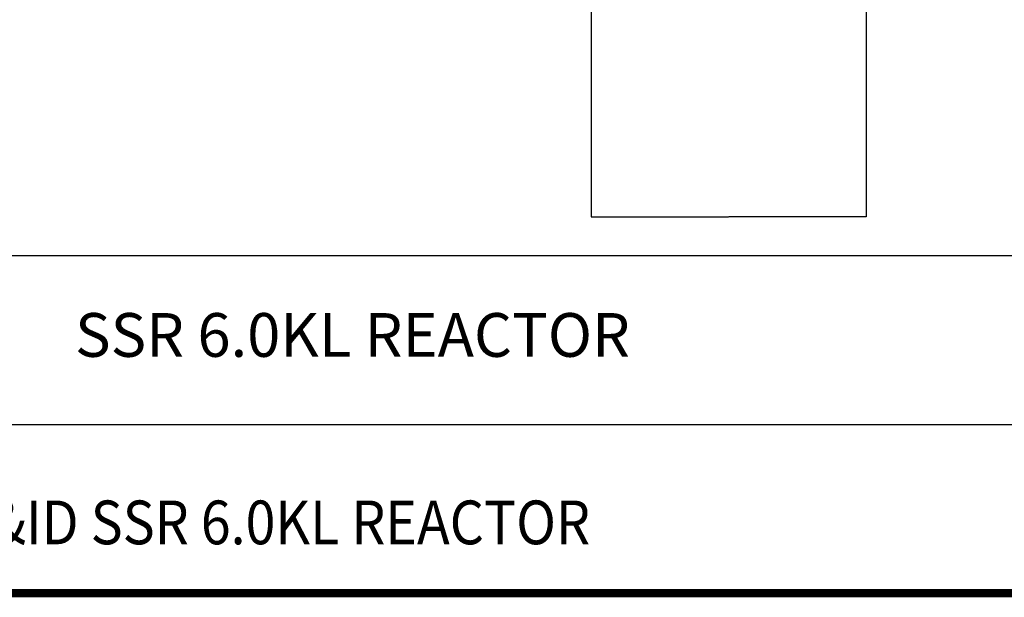
# Model space of a CAD drawing. Units: millimetres. Extents: x 353872 to 441597, y 126154 to 187356.
# Tile 5 of 28: x 381210 to 399262, y 126840 to 137428. Entities that reach past the tile are written whole.
import ezdxf

# ---------------------------------------------------------------- set-up
doc = ezdxf.new("R2010")
doc.units = ezdxf.units.MM
for name, color, linetype, lineweight in [('A-ANNO-DIMS', 2, 'Continuous', 18), ('P-ANNO-TEXT', 7, 'Continuous', 25), ('P-ANNO-TTLB', 7, 'Continuous', 25)]:
    doc.layers.add(name, color=color, linetype=linetype, lineweight=lineweight)
doc.styles.add('ROMANT', font='romant.shx', dxfattribs={"width": 0.8, "height": 3.5})
doc.styles.get("Standard").update_dxf_attribs({"font": 'arial.ttf'})
doc.dimstyles.get("Standard").update_dxf_attribs({"dimtxt": 0.18, "dimasz": 0.18, "dimexe": 0.18, "dimexo": 0.0625, "dimgap": 0.09, "dimtad": 0, "dimtih": 1, "dimtoh": 1, "dimdec": 4, "dimzin": 0, "dimdsep": 46, "dimtxsty": 'Standard', "dimcen": 0.09, "dimadec": 0, "dimazin": 0, "dimtfac": 1, "dimtdec": 4, "dimtofl": 0, "dimtmove": 0, "dimatfit": 3, "dimfxl": 1, "dimtolj": 1, "dimtzin": 0, "dimarcsym": 0})

# ---------------------------------------------------------------- blocks, each defined once
blk = doc.blocks.new('*D29')
at = {"layer": 'A-ANNO-DIMS', "color": 0, "lineweight": -2, "transparency": 16777216}
for p, q in [((391690, 148464), (391690, 133813)), ((396728, 148464), (396728, 133813)), ((391690, 133813), (394208, 133813)), ((396727, 133813), (394209, 133813))]:
    blk.add_line(p, q, dxfattribs=at)
at = {"layer": 'A-ANNO-DIMS', "color": 0, "transparency": 16777216}
for points in [[(391690, 133813), (391690, 133813), (391690, 133813)], [(396727, 133813), (396727, 133813), (396728, 133813)]]:
    blk.add_solid(points, dxfattribs=at)
at = {"layer": 'Defpoints', "color": 0, "transparency": 16777216}
for p in [(391690, 148465), (396728, 148465), (396728, 133813)]:
    blk.add_point(p, dxfattribs=at)
at = {"layer": 'A-ANNO-DIMS', "color": 0, "transparency": 16777216, "insert": (394209, 133813), "char_height": 0.18, "attachment_point": 5}
blk.add_mtext('\\A1;5038', dxfattribs=at)

msp = doc.modelspace()

# ---------------------------------------------------------------- linework, layer by layer
at = {"layer": 'P-ANNO-TTLB'}
for p, q in [((353948.03, 133103.92), (440835.19, 133103.92)), ((371550.6, 130010.13), (440835.19, 130010.13))]:
    msp.add_line(p, q, dxfattribs=at)
at = {"layer": 'P-ANNO-TTLB', "const_width": 152.43}
msp.add_lwpolyline([(353948.03, 187280.05), (353948.03, 126916.34), (440835.19, 126916.34), (440835.19, 187280.05)], close=True, dxfattribs=at)

# ---------------------------------------------------------------- texts
at = {"layer": 'P-ANNO-TEXT', "style": 'ROMANT'}
msp.add_text('SSR 6.0KL REACTOR', height=802.0939, dxfattribs=at).set_placement((382224.6, 131248.2))
at = {"layer": 'P-ANNO-TEXT', "style": 'ROMANT', "width": 0.9}
msp.add_text('P&ID SSR 6.0KL REACTOR', height=802.0939, dxfattribs=at).set_placement((380031.07, 127811.87))

# ---------------------------------------------------------------- dimensions: what is measured, and where the dimension line sits
at = {"layer": 'A-ANNO-DIMS'}
dim = msp.add_linear_dim(base=(396727.53, 133812.84), p1=(391689.9, 148464.52), p2=(396727.53, 148464.52), dimstyle='Standard', override={"dimdec": 0, "dimlfac": 1, "dimrnd": 0, "dimzin": 0, "dimdsep": 46, "dimlunit": 2}, dxfattribs=at)
dim.commit()
dim.dimension.update_dxf_attribs({"geometry": '*D29', "text_midpoint": (394208.72, 133812.84)})

doc.saveas('drawing.dxf')
